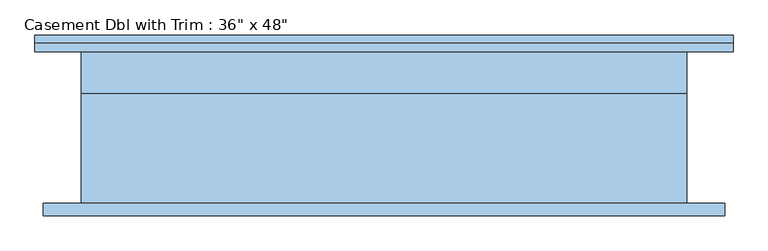
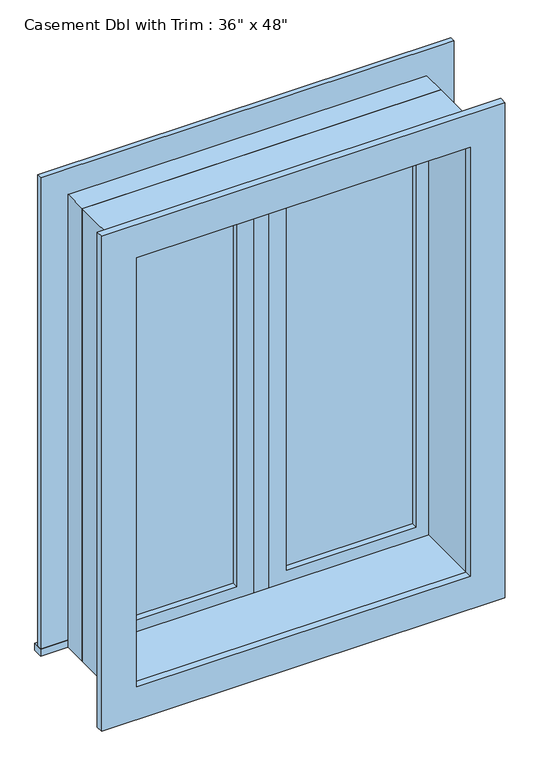
"""IFC4 building model written with IfcOpenShell, lengths in millimetres: window geometry."""

from ifc_helpers import new_model, si_unit, frame, origin, place, context, project, spatial, polyline, outline, extrude, source, transform, mapped, element, save


def window_419b5846(model_context):
    return source(origin(), model_context, "Body", "SweptSolid", [
        extrude(outline(polyline([(63.5, 98.425), (393.7, 98.425), (393.7, 85.725), (63.5, 85.725), (63.5, 98.425)])), frame((0.0, 0.0, 977.9), z_axis=(0.0, 0.0, 1.0), x_axis=(1.0, 0.0, 0.0)), (0.0, 0.0, 1.0), 1092.2),
        extrude(outline(polyline([(2114.55, 19.05), (933.45, 19.05), (933.45, 438.15), (2114.55, 438.15), (2114.55, 19.05)]), holes=[polyline([(2070.1, 63.5), (2070.1, 393.7), (977.9, 393.7), (977.9, 63.5), (2070.1, 63.5)])]), frame((0.0, 69.85, 0.0), z_axis=(0.0, 1.0, 0.0), x_axis=(0.0, 0.0, 1.0)), (0.0, 0.0, 1.0), 44.45),
        extrude(outline(polyline([(19.05, 69.85), (-19.05, 69.85), (-19.05, 133.35), (19.05, 133.35), (19.05, 69.85)])), frame((0.0, 0.0, 933.45), z_axis=(0.0, 0.0, 1.0), x_axis=(1.0, 0.0, 0.0)), (0.0, 0.0, 1.0), 1181.1),
        extrude(outline(polyline([(-527.05, 158.75), (527.05, 158.75), (527.05, 133.35), (-527.05, 133.35), (-527.05, 158.75)])), frame((0.0, 0.0, 914.4), z_axis=(0.0, 0.0, 1.0), x_axis=(1.0, 0.0, 0.0)), (0.0, 0.0, 1.0), 19.05),
        extrude(outline(polyline([(2114.55, -438.15), (2114.55, 438.15), (933.45, 438.15), (933.45, 527.05), (2203.45, 527.05), (2203.45, -527.05), (933.45, -527.05), (933.45, -438.15), (2114.55, -438.15)])), frame((0.0, 133.35, 0.0), z_axis=(0.0, 1.0, 0.0), x_axis=(0.0, 0.0, 1.0)), (0.0, 0.0, 1.0), 12.7),
        extrude(outline(polyline([(2190.75, 514.35), (2190.75, -514.35), (857.25, -514.35), (857.25, 514.35), (2190.75, 514.35)]), holes=[polyline([(2101.85, 425.45), (946.15, 425.45), (946.15, -425.45), (2101.85, -425.45), (2101.85, 425.45)])]), frame((0.0, -114.3, 0.0), z_axis=(0.0, 1.0, 0.0), x_axis=(0.0, 0.0, 1.0)), (0.0, 0.0, 1.0), 19.05),
        extrude(outline(polyline([(-63.5, 85.725), (-393.7, 85.725), (-393.7, 98.425), (-63.5, 98.425), (-63.5, 85.725)])), frame((0.0, 0.0, 977.9), z_axis=(0.0, 0.0, 1.0), x_axis=(1.0, 0.0, 0.0)), (0.0, 0.0, 1.0), 1092.2),
        extrude(outline(polyline([(2114.55, -438.15), (933.45, -438.15), (933.45, -19.05), (2114.55, -19.05), (2114.55, -438.15)]), holes=[polyline([(2070.1, -393.7), (2070.1, -63.5), (977.9, -63.5), (977.9, -393.7), (2070.1, -393.7)])]), frame((0.0, 69.85, 0.0), z_axis=(0.0, 1.0, 0.0), x_axis=(0.0, 0.0, 1.0)), (0.0, 0.0, 1.0), 44.45),
        extrude(outline(polyline([(2133.6, -457.2), (914.4, -457.2), (914.4, 457.2), (2133.6, 457.2), (2133.6, -457.2)]), holes=[polyline([(2101.85, -425.45), (2101.85, 425.45), (946.15, 425.45), (946.15, -425.45), (2101.85, -425.45)])]), frame((0.0, -95.25, 0.0), z_axis=(0.0, 1.0, 0.0), x_axis=(0.0, 0.0, 1.0)), (0.0, 0.0, 1.0), 165.1),
        extrude(outline(polyline([(2133.6, 457.2), (2133.6, -457.2), (914.4, -457.2), (914.4, 457.2), (2133.6, 457.2)]), holes=[polyline([(2114.55, 438.15), (933.45, 438.15), (933.45, -438.15), (2114.55, -438.15), (2114.55, 438.15)])]), frame((0.0, 69.85, 0.0), z_axis=(0.0, 1.0, 0.0), x_axis=(0.0, 0.0, 1.0)), (0.0, 0.0, 1.0), 63.5),
    ])


if __name__ == "__main__":
    model = new_model("IFC4")
    model_context = context("Model", 3, world=origin())
    ifc_project = project(units=[si_unit("LENGTHUNIT", "METRE", prefix="MILLI")], contexts=[model_context])
    site = spatial("IfcSite", under=ifc_project)
    building = spatial("IfcBuilding", under=site)
    placement = place(None, origin())
    window_shape = window_419b5846(model_context)
    element("IfcWindow", 1, ObjectType="Casement Dbl with Trim : 36\" x 48\"", at=placement, inside=building, context=model_context, shape_type="MappedRepresentation", body=[
        mapped(window_shape, transform((0.0, 0.0, 0.0), x_axis=(1.0, 0.0, 0.0), y_axis=(0.0, 1.0, 0.0), z_axis=(0.0, 0.0, 1.0))),
    ])
    save(model, "model.ifc")

# Revit data of these elements
# Type "Casement Dbl with Trim : 36\" x 48\""
#   Type Mark = "19"
#   Construction Type Id = "GSP4R"
#   Assembly Code = "B2020100"
#   Analytic Construction = "1/8 in Pilkington single glazing"
#   Visual Light Transmittance = 0.9
#   Solar Heat Gain Coefficient = 0.78
#   Heat Transfer Coefficient (U) = 0.6496 BTU/(h·ft²·°F)
#   Height = 4' - 0"
#   Default Sill Height = 3' - 0"
#   Trim Projection - Ext. = 0' - 0 1/2"
#   Trim Projection - Int. = 0' - 0 3/4"
#   Trim Width - Exterior = 0' - 3 1/2"
#   Trim Width - Interior = 0' - 3 1/2"
#   Width = 3' - 0"
#   Window Inset = 0' - 0 3/4"
#   Define Thermal Properties by = 1
#   Glass Pane Material = Glass
#   Sash Material = Sash
#   Trim Exterior Material = Trim
#   Trim Interior Material = Trim
#   Wall Closure = (empty or 0)
# Element 1 (IfcWindow, "Casement Dbl with Trim : 36\" x 48\"")
#   Materials on its faces: "Sash", "Trim", "Glass"
# Materials
#   "Glass": class "Glass", colour RGB 0 128 192, transparency 0.75, Description = "Soda Lime Glass", Cost = 0
#   "Sash": class "Wood", colour RGB 224 178 126, transparency 0
#   "Trim": class "Wood", colour RGB 224 178 126, transparency 0
